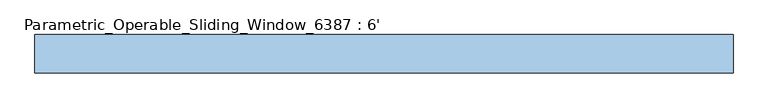
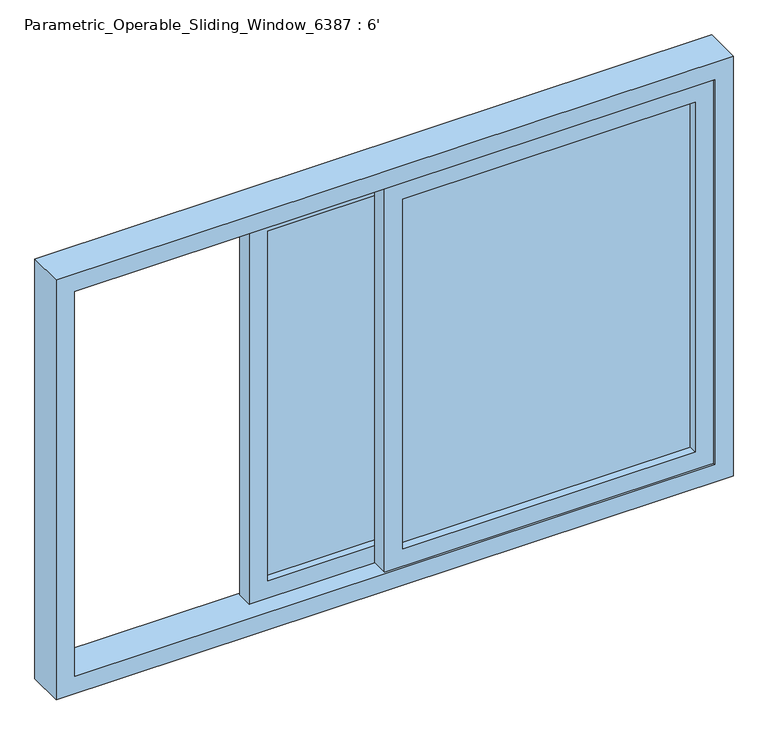
"""IFC4 building model written with IfcOpenShell, lengths in millimetres: window geometry, Parametric_Operable_Sliding_Window_6387 : 6'."""

from ifc_helpers import new_model, si_unit, frame, origin, place, context, project, spatial, polyline, outline, extrude, source, transform, mapped, element, save


def parametric_operable_sliding_window_6387_6_8dd7d652(model_context):
    return source(origin(), model_context, "Body", "SweptSolid", [
        extrude(outline(polyline([(900.0, 1174.4), (2100.0, 1174.4), (2100.0, -654.4), (900.0, -654.4), (900.0, 1174.4)]), holes=[polyline([(2050.0, -604.4), (2050.0, 1124.4), (950.0, 1124.4), (950.0, -604.4), (2050.0, -604.4)])]), frame((0.0, -50.0, 0.0), z_axis=(0.0, 1.0, 0.0), x_axis=(0.0, 0.0, 1.0)), (0.0, 0.0, 1.0), 100.0),
        extrude(outline(polyline([(2050.0, 235.0), (950.0, 235.0), (950.0, 1124.4), (2050.0, 1124.4), (2050.0, 235.0)]), holes=[polyline([(2000.0, 285.0), (2000.0, 1074.4), (1000.0, 1074.4), (1000.0, 285.0), (2000.0, 285.0)])]), frame((0.0, -45.0, 0.0), z_axis=(0.0, 1.0, 0.0), x_axis=(0.0, 0.0, 1.0)), (0.0, 0.0, 1.0), 45.0),
        extrude(outline(polyline([(1074.4, -16.5), (1074.4, -22.5), (285.0, -22.5), (285.0, -16.5), (1074.4, -16.5)])), frame((0.0, 0.0, 1000.0), z_axis=(0.0, 0.0, 1.0), x_axis=(1.0, 0.0, 0.0)), (0.0, 0.0, 1.0), 1000.0),
        extrude(outline(polyline([(2050.0, -104.4), (950.0, -104.4), (950.0, 785.0), (2050.0, 785.0), (2050.0, -104.4)]), holes=[polyline([(1000.0, -54.4), (2000.0, -54.4), (2000.0, 735.0), (1000.0, 735.0), (1000.0, -54.4)])]), frame((0.0, 0.0, 0.0), z_axis=(0.0, 1.0, 0.0), x_axis=(0.0, 0.0, 1.0)), (0.0, 0.0, 1.0), 45.0),
        extrude(outline(polyline([(-54.4, 25.5), (735.0, 25.5), (735.0, 19.5), (-54.4, 19.5), (-54.4, 25.5)])), frame((0.0, 0.0, 1000.0), z_axis=(0.0, 0.0, 1.0), x_axis=(1.0, 0.0, 0.0)), (0.0, 0.0, 1.0), 1000.0),
    ])


if __name__ == "__main__":
    model = new_model("IFC4")
    model_context = context("Model", 3, world=origin())
    ifc_project = project(units=[si_unit("LENGTHUNIT", "METRE", prefix="MILLI")], contexts=[model_context])
    site = spatial("IfcSite", under=ifc_project)
    building = spatial("IfcBuilding", under=site)
    placement = place(None, origin())
    parametric_operable_sliding_window_6387_6_shape = parametric_operable_sliding_window_6387_6_8dd7d652(model_context)
    element("IfcWindow", 1, ObjectType="Parametric_Operable_Sliding_Window_6387 : 6'", at=placement, inside=building, context=model_context, shape_type="MappedRepresentation", body=[
        mapped(parametric_operable_sliding_window_6387_6_shape, transform((0.0, 0.0, 0.0), x_axis=(1.0, 0.0, 0.0), y_axis=(0.0, 1.0, 0.0), z_axis=(0.0, 0.0, 1.0))),
    ])
    save(model, "model.ifc")

# Revit data of these elements
# Type "Parametric_Operable_Sliding_Window_6387 : 6'"
#   Type Mark = "61"
#   Sash Offset From Frame = 0' - 0"
#   Sash Width = 0' - 3.54331"
#   Sash Thickness = 0' - 1.9685"
#   Sash Edge Offset = 0' - 0.19685"
#   Rough Tolerance = 0' - 0.3937"
#   Rough Width = 6' - 1.33858"
#   Rough Height = 4' - 0.58268"
#   Reveal Thickness = 0' - 0.47244"
#   Panel Sash Depth = 0' - 1.77165"
#   Pane Width = 2' - 11.01575"
#   Pane Height = 3' - 7.30709"
#   Opened Pane Portion [instance default] = 1' - 7.68504"
#   Glass Thickness = 0' - 0.23622"
#   Frame Offset = 0' - 0"
#   Height = 3' - 11.24409"
#   Frame Width = 0' - 3.93701"
#   Frame Thickness = 0' - 1.9685"
#   Frame Sill = 0' - 0.98425"
#   Width = 6' - 0"
#   Default Sill Height = 2' - 11.43307"
#   Architrave Width = 0' - 2.67717"
#   Architrave Thickness = 0' - 0.47244"
#   Architrave Offset = 0' - 0.19685"
#   Show Reveal = no
#   Show Architrave = no
#   Reveal = Window Reveal
#   Glass = Window Glass
#   Frame = Window Frame
#   Architrave = Window Architrave
#   Wall Closure = (empty or 0)
#   Assembly Code = ""
# Element 1 (IfcWindow, "Parametric_Operable_Sliding_Window_6387 : 6'")
#   Materials on its faces: "Window Frame", "Window Glass"
# Materials
#   "Window Reveal": colour RGB 255 255 255, transparency 0
#   "Window Glass": colour RGB 0 0 255, transparency 0.75
#   "Window Frame": colour RGB 249 249 249, transparency 0, Keynote = "L10", Cost = 0
#   "Window Architrave": colour RGB 255 255 255, transparency 0
